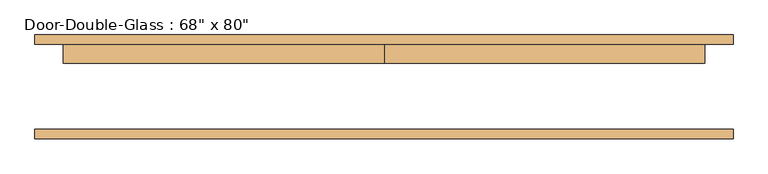
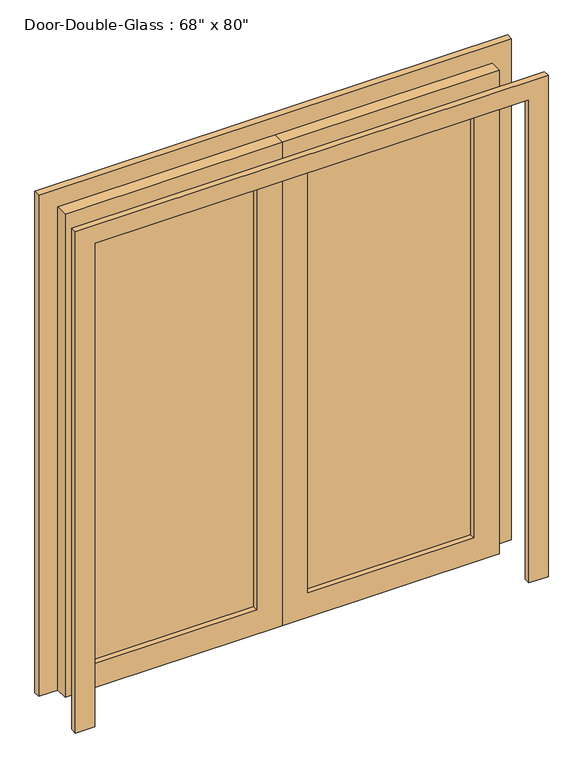
"""IFC4 building model written with IfcOpenShell, lengths in millimetres: door geometry."""

from ifc_helpers import new_model, si_unit, frame, origin, place, context, project, spatial, polyline, outline, extrude, source, transform, mapped, element, save


def door_423d55ee(model_context):
    return source(origin(), model_context, "Body", "SweptSolid", [
        extrude(outline(polyline([(2032.0, -863.6), (0.0, -863.6), (0.0, 0.0), (2032.0, 0.0), (2032.0, -863.6)]), holes=[polyline([(1930.4, -762.0), (1930.4, -101.6), (101.6, -101.6), (101.6, -762.0), (1930.4, -762.0)])]), frame((0.0, 65.88125, 0.0), z_axis=(0.0, 1.0, 0.0), x_axis=(0.0, 0.0, 1.0)), (0.0, 0.0, 1.0), 50.8),
        extrude(outline(polyline([(2032.0, 863.6), (2032.0, 0.0), (0.0, 0.0), (0.0, 863.6), (2032.0, 863.6)]), holes=[polyline([(1930.4, 762.0), (101.6, 762.0), (101.6, 101.6), (1930.4, 101.6), (1930.4, 762.0)])]), frame((0.0, 65.88125, 0.0), z_axis=(0.0, 1.0, 0.0), x_axis=(0.0, 0.0, 1.0)), (0.0, 0.0, 1.0), 50.8),
        extrude(outline(polyline([(101.6, 94.45625), (762.0, 94.45625), (762.0, 88.10625), (101.6, 88.10625), (101.6, 94.45625)])), frame((0.0, 0.0, 101.6), z_axis=(0.0, 0.0, 1.0), x_axis=(1.0, 0.0, 0.0)), (0.0, 0.0, 1.0), 1828.8),
        extrude(outline(polyline([(-762.0, 94.45625), (-101.6, 94.45625), (-101.6, 88.10625), (-762.0, 88.10625), (-762.0, 94.45625)])), frame((0.0, 0.0, 101.6), z_axis=(0.0, 0.0, 1.0), x_axis=(1.0, 0.0, 0.0)), (0.0, 0.0, 1.0), 1828.8),
        extrude(outline(polyline([(0.0, 939.8), (2108.2, 939.8), (2108.2, -939.8), (0.0, -939.8), (0.0, -863.6), (2032.0, -863.6), (2032.0, 863.6), (0.0, 863.6), (0.0, 939.8)])), frame((0.0, 116.68125, 0.0), z_axis=(0.0, 1.0, 0.0), x_axis=(0.0, 0.0, 1.0)), (0.0, 0.0, 1.0), 25.4),
        extrude(outline(polyline([(0.0, 939.8), (2108.2, 939.8), (2108.2, -939.8), (0.0, -939.8), (0.0, -863.6), (2032.0, -863.6), (2032.0, 863.6), (0.0, 863.6), (0.0, 939.8)])), frame((0.0, -137.31875, 0.0), z_axis=(0.0, 1.0, 0.0), x_axis=(0.0, 0.0, 1.0)), (0.0, 0.0, 1.0), 25.4),
    ])


if __name__ == "__main__":
    model = new_model("IFC4")
    model_context = context("Model", 3, world=origin())
    ifc_project = project(units=[si_unit("LENGTHUNIT", "METRE", prefix="MILLI")], contexts=[model_context])
    site = spatial("IfcSite", under=ifc_project)
    building = spatial("IfcBuilding", under=site)
    placement = place(None, origin())
    door_shape = door_423d55ee(model_context)
    element("IfcDoor", 1, ObjectType="Door-Double-Glass : 68\" x 80\"", at=placement, inside=building, context=model_context, shape_type="MappedRepresentation", body=[
        mapped(door_shape, transform((0.0, 0.0, 0.0), x_axis=(1.0, 0.0, 0.0), y_axis=(0.0, 1.0, 0.0), z_axis=(0.0, 0.0, 1.0))),
    ])
    save(model, "model.ifc")

# Revit data of these elements
# Type "Door-Double-Glass : 68\" x 80\""
#   Type Mark = "8"
#   Construction Type Id = "opn-d45"
#   Assembly Code = "C1020"
#   Analytic Construction = "Wood frame, double glass door "
#   W = 2' - 10"
#   Thickness = 0' - 2"
#   Thermal Resistance (R) = 1.8150 (h·ft²·°F)/BTU
#   Swing Angle [instance default] = 90.00°
#   Heat Transfer Coefficient (U) = 0.5510 BTU/(h·ft²·°F)
#   Height = 6' - 8"
#   Bottom Rail = 0' - 4"
#   Top Rail = 0' - 4"
#   Stiles = 0' - 4"
#   Trim Projection = 0' - 1"
#   Trim Width = 0' - 3"
#   Width = 5' - 8"
#   Define Thermal Properties by = 1
#   Glazing = Glass
#   Panel Material = Wood - Birch - Solid Stained Light Low Gloss
#   Trim Material = Paint - Sienna
#   Visual Light Transmittance = 0
#   Solar Heat Gain Coefficient = 0
#   Function = (empty or 0)
#   Wall Closure = (empty or 0)
# Element 1 (IfcDoor, "Door-Double-Glass : 68\" x 80\"")
#   Materials on its faces: "Wood - Birch - Solid Stained Light Low Gloss", "Paint - Sienna", "Glass"
# Materials
#   "Glass": class "Glass", colour RGB 0 128 192, transparency 0.75, Description = "Soda Lime Glass", Cost = 0
#   "Wood - Birch - Solid Stained Light Low Gloss": class "Wood", colour RGB 210 159 95, transparency 0, Cost = 0
#   "Paint - Sienna": colour RGB 118 70 51, transparency 0, Cost = 0
